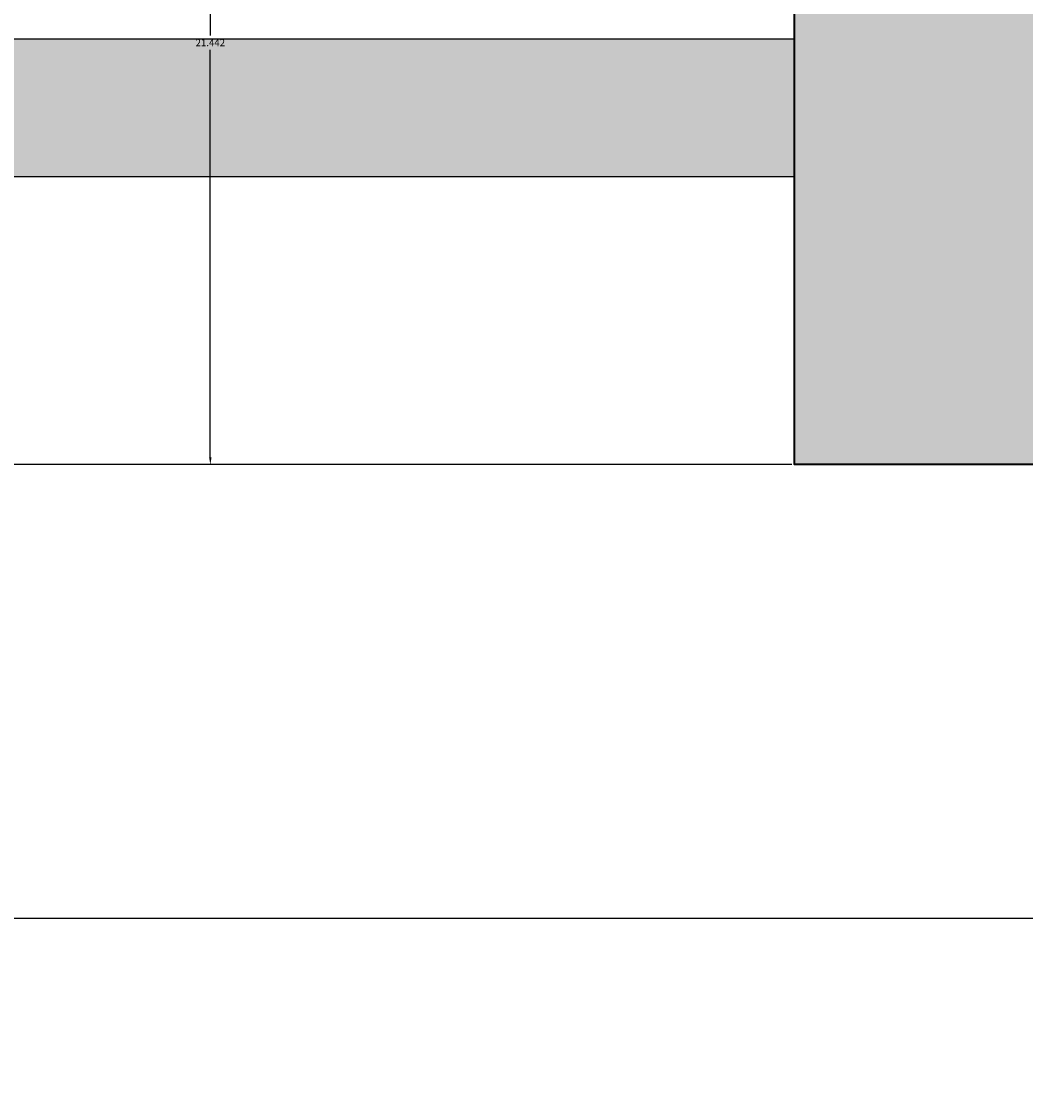
# Model space of a CAD drawing. Units: millimetres. Extents: x -11 to 280, y -4 to 208.
# Tile 49 of 55: x 186 to 211, y 129 to 156. Entities that reach past the tile are written whole.
import ezdxf

# ---------------------------------------------------------------- set-up
doc = ezdxf.new("R2010")
doc.units = ezdxf.units.MM
for name, color, linetype, lineweight in [('M-DIMS', 2, 'Continuous', 18), ('M-HYDR-EQPM', 7, 'Continuous', 35), ('M-HYDR-EQPM-PATT', 252, 'Continuous', 13), ('M-HYDR-SUCT', 7, 'Continuous', 25)]:
    doc.layers.add(name, color=color, linetype=linetype, lineweight=lineweight)
doc.layers.add('M-HYDR-SUCT-PATT', color=221, linetype='Continuous', lineweight=13, true_color=0xff7fdf)
doc.styles.get("Standard").update_dxf_attribs({"font": 'arial.ttf'})
doc.dimstyles.get("Standard").update_dxf_attribs({"dimtxt": 0.18, "dimasz": 0.18, "dimexe": 0.18, "dimexo": 0.0625, "dimgap": 0.09, "dimtad": 0, "dimtih": 1, "dimtoh": 1, "dimdec": 4, "dimzin": 0, "dimdsep": 46, "dimtxsty": 'Standard', "dimcen": 0.09, "dimadec": 0, "dimazin": 0, "dimtfac": 1, "dimtdec": 4, "dimtofl": 0, "dimtmove": 0, "dimatfit": 3, "dimfxl": 1, "dimtolj": 1, "dimtzin": 0, "dimarcsym": 0})

# ---------------------------------------------------------------- blocks, each defined once
blk = doc.blocks.new('*D5')
at = {"layer": 'Defpoints', "color": 0, "transparency": 16777216}
for p in [(24.759, 192.645), (-10.087, 11.435), (261.686, 11.435)]:
    blk.add_point(p, dxfattribs=at)
at = {"layer": 'M-DIMS', "color": 0, "lineweight": -2, "transparency": 16777216}
for p, q in [((24.696, 192.645), (-10.267, 192.645)), ((-10.087, 192.465), (-10.087, 102.222)), ((-10.087, 11.615), (-10.087, 101.858)), ((261.624, 11.435), (-10.267, 11.435))]:
    blk.add_line(p, q, dxfattribs=at)
at = {"layer": 'M-DIMS', "color": 0, "transparency": 16777216}
for points in [[(-10.117, 192.465), (-10.057, 192.465), (-10.087, 192.645)], [(-10.117, 11.615), (-10.057, 11.615), (-10.087, 11.435)]]:
    blk.add_solid(points, dxfattribs=at)
at = {"layer": 'M-DIMS', "color": 0, "transparency": 16777216, "insert": (-10.087, 102.04), "char_height": 0.18, "attachment_point": 5}
blk.add_mtext('\\A1;181.2', dxfattribs=at)
blk = doc.blocks.new('*D14')
at = {"layer": 'Defpoints', "color": 0, "transparency": 16777216}
for p in [(-10.087, 144.661), (205.531, 144.661), (226.511, 133.123)]:
    blk.add_point(p, dxfattribs=at)
at = {"layer": 'M-DIMS', "color": 0, "lineweight": -2, "transparency": 16777216}
for p, q in [((205.469, 144.661), (-10.267, 144.661)), ((-10.087, 144.481), (-10.087, 139.074)), ((-10.087, 133.303), (-10.087, 138.71)), ((226.448, 133.123), (-10.267, 133.123))]:
    blk.add_line(p, q, dxfattribs=at)
at = {"layer": 'M-DIMS', "color": 0, "transparency": 16777216}
for points in [[(-10.117, 144.481), (-10.057, 144.481), (-10.087, 144.661)], [(-10.117, 133.303), (-10.057, 133.303), (-10.087, 133.123)]]:
    blk.add_solid(points, dxfattribs=at)
at = {"layer": 'M-DIMS', "color": 0, "transparency": 16777216, "insert": (-10.087, 138.892), "char_height": 0.18, "attachment_point": 5}
blk.add_mtext('\\A1;11.538', dxfattribs=at)
blk = doc.blocks.new('*D20')
at = {"layer": 'Defpoints', "color": 0, "transparency": 16777216}
for p in [(231.68, 207.495), (151.022, 43.599), (231.68, 43.599)]:
    blk.add_point(p, dxfattribs=at)
at = {"layer": 'M-DIMS', "color": 0, "lineweight": -2, "transparency": 16777216}
for p, q in [((151.022, 43.662), (151.022, 207.675)), ((151.202, 207.495), (190.957, 207.495)), ((231.5, 207.495), (191.745, 207.495)), ((231.68, 43.662), (231.68, 207.675))]:
    blk.add_line(p, q, dxfattribs=at)
at = {"layer": 'M-DIMS', "color": 0, "transparency": 16777216}
for points in [[(151.202, 207.525), (151.202, 207.465), (151.022, 207.495)], [(231.5, 207.525), (231.5, 207.465), (231.68, 207.495)]]:
    blk.add_solid(points, dxfattribs=at)
at = {"layer": 'M-DIMS', "color": 0, "transparency": 16777216, "insert": (191.351, 207.495), "char_height": 0.18, "attachment_point": 5}
blk.add_mtext('\\A1;80.66', dxfattribs=at)
blk = doc.blocks.new('*D26')
at = {"layer": 'Defpoints', "color": 0, "transparency": 16777216}
for p in [(190.681, 166.103), (205.531, 166.103), (205.531, 144.661)]:
    blk.add_point(p, dxfattribs=at)
at = {"layer": 'M-DIMS', "color": 0, "lineweight": -2, "transparency": 16777216}
for p, q in [((205.469, 166.103), (190.501, 166.103)), ((190.681, 165.923), (190.681, 155.562)), ((190.681, 144.841), (190.681, 155.202)), ((205.469, 144.661), (190.501, 144.661))]:
    blk.add_line(p, q, dxfattribs=at)
at = {"layer": 'M-DIMS', "color": 0, "transparency": 16777216}
for points in [[(190.651, 165.923), (190.711, 165.923), (190.681, 166.103)], [(190.651, 144.841), (190.711, 144.841), (190.681, 144.661)]]:
    blk.add_solid(points, dxfattribs=at)
at = {"layer": 'M-DIMS', "color": 0, "transparency": 16777216, "insert": (190.681, 155.382), "char_height": 0.18, "attachment_point": 5}
blk.add_mtext('\\A1;21.442', dxfattribs=at)

msp = doc.modelspace()

# ---------------------------------------------------------------- hatches: boundary and pattern name
at = {"layer": 'M-HYDR-EQPM-PATT'}
h = msp.add_hatch(color=256, dxfattribs=at)
h.set_gradient(color1=(248, 153, 30), color2=(248, 153, 30), tint=1)
h.paths.add_polyline_path([(236.9353, 165.103), (205.5315, 165.103), (205.5315, 144.6609), (236.9353, 144.6609)])
h.paths.add_polyline_path([(244.8074, 166.103), (205.5315, 166.103), (205.5315, 165.103), (236.9353, 165.103), (245.4299, 165.103)])
h.paths.add_polyline_path([(248.3313, 165.603, -0.4142136), (248.8313, 166.103), (245.9853, 166.103), (246.6078, 165.103), (248.8313, 165.103, -0.4142136)])
h.paths.add_polyline_path([(249.3313, 165.603, 1), (248.3313, 165.603, 0.4142136), (248.8313, 165.103, 0.4142136)])
at = {"layer": 'M-HYDR-SUCT-PATT'}
h = msp.add_hatch(color=256, dxfattribs=at)
h.set_gradient(color1=(255, 127, 223), color2=(255, 127, 223), tint=1, name='INVCYLINDER')
h.paths.add_polyline_path([(91.3629, 155.4768), (91.3629, 132.4768), (58.3629, 132.4768), (58.3629, 153.9768), (54.8629, 153.9768), (54.8629, 128.9768), (94.8629, 128.9768), (94.8629, 151.9768), (205.5315, 151.9768), (205.5315, 155.4768)])
h.paths.add_polyline_path([(91.3, 114.9452, 1), (78.8273, 114.9452), (78.8273, 108.8141), (42.6453, 108.8141), (42.6453, 153.9768), (39.1453, 153.9768), (39.1453, 105.3141), (78.8273, 105.3141), (78.8273, 98.1491, 1), (91.3, 98.1491), (91.3, 105.3141), (95.5776, 105.3141), (95.5776, 108.8141), (91.3, 108.8141)])
h.paths.add_polyline_path([(228.7, 138.4081), (232.2, 138.4081), (232.2, 144.6609), (228.7, 144.6609)])
h.paths.add_polyline_path([(253.1005, 151.9768, 1), (253.1005, 155.4768), (252.6001, 155.4768), (253.5249, 153.991, -0.1401047), (253.6005, 153.7268, -0.7542249), (252.676, 153.4626), (251.4221, 155.4768), (236.9353, 155.4768), (236.9353, 151.9768)])
h.paths.add_polyline_path([(30.8182, 40.7626), (30.8182, 36.7626), (60.8182, 36.7626), (60.8182, 40.7626)])

# ---------------------------------------------------------------- linework, layer by layer
at = {"layer": 'M-HYDR-EQPM'}
msp.add_lwpolyline([(205.5315, 165.103), (236.9353, 165.103), (236.9353, 144.6609), (205.5315, 144.6609)], close=True, dxfattribs=at)
at = {"layer": 'M-HYDR-SUCT'}
for points in [[(58.3629, 153.9768), (58.3629, 132.4768), (91.3629, 132.4768), (91.3629, 155.4768), (205.5315, 155.4768)], [(54.8629, 153.9768), (54.8629, 128.9768), (94.8629, 128.9768), (94.8629, 151.9768), (205.5315, 151.9768)]]:
    msp.add_lwpolyline(points, dxfattribs=at)

# ---------------------------------------------------------------- dimensions: what is measured, and where the dimension line sits
at = {"layer": 'M-DIMS'}
dim = msp.add_linear_dim(base=(231.6803, 207.495), p1=(151.0217, 43.5991), p2=(231.6803, 43.5991), dimstyle='Standard', override={"dimdec": 2, "dimlfac": 1, "dimrnd": 0, "dimzin": 0, "dimdsep": 46, "dimlunit": 2}, dxfattribs=at)
dim.commit()
dim.dimension.update_dxf_attribs({"geometry": '*D20', "text_midpoint": (191.351, 207.495)})
for base, p1, p2, override, picture, middle in [((-10.0865, 11.4346), (24.7588, 192.645), (261.6863, 11.4346), {"dimdec": 1, "dimlfac": 1, "dimrnd": 0, "dimzin": 0, "dimdsep": 46, "dimlunit": 2}, '*D5', (-10.0865, 102.0398)), ((190.6815, 166.103), (205.5315, 144.6609), (205.5315, 166.103), {"dimdec": 3, "dimlfac": 1, "dimrnd": 0, "dimzin": 0, "dimdsep": 46, "dimlunit": 2}, '*D26', (190.6815, 155.382)), ((-10.0865, 144.6609), (226.5106, 133.1228), (205.5315, 144.6609), {"dimdec": 3, "dimlfac": 1, "dimrnd": 0, "dimzin": 0, "dimdsep": 46, "dimlunit": 2}, '*D14', (-10.0865, 138.8918))]:
    dim = msp.add_linear_dim(base=base, p1=p1, p2=p2, angle=90, dimstyle='Standard', override=override, dxfattribs=at)
    dim.commit()
    dim.dimension.update_dxf_attribs({"geometry": picture, "text_midpoint": middle})

doc.saveas('drawing.dxf')
